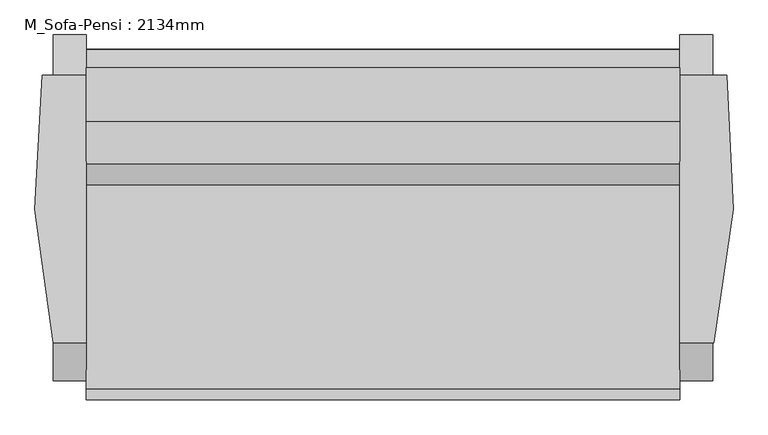
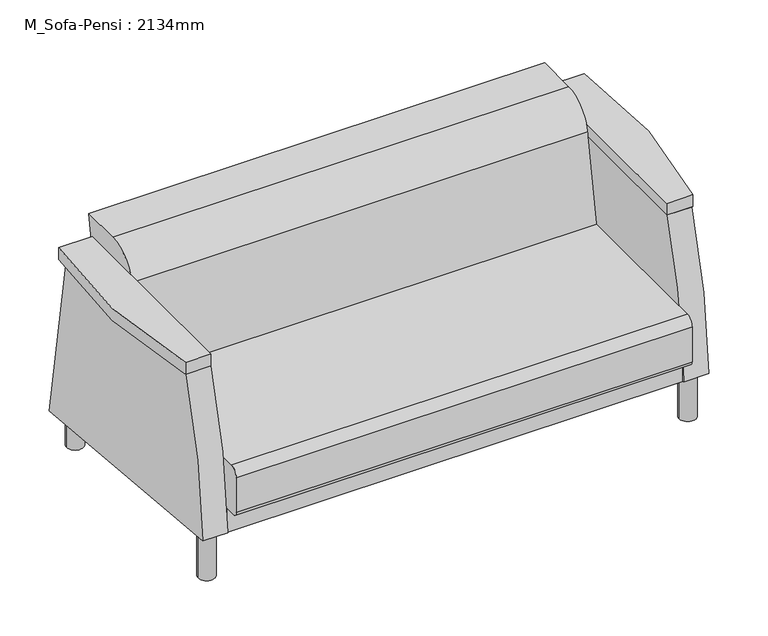
"""IFC4 building model written with IfcOpenShell, lengths in millimetres: furniture geometry, M_Sofa-Pensi : 2134mm."""

from ifc_helpers import new_model, si_unit, point, frame, frame_2d, origin, origin_with_axes, place, context, project, spatial, polyline, circle_curve, trimmed, segment, composite_curve, outline, extrude, source, transform, mapped, element, save
from ifc_brep_helpers import plane_surface, cylinder_surface, advanced_brep


def m_sofa_pensi_2134mm_8f487940(model_context):
    return source(origin(), model_context, "Body", "SolidModel", [
        advanced_brep(
        [(1040.60625, 701.7619204, 79.3588346), (1040.60625, 608.6917937, 626.0203985), (1040.60625, -9.3943348, 626.0203985), (1040.60625, -97.7900405, 149.3105671), (964.40625, -9.3943348, 626.0203985), (964.40625, 608.6917937, 626.0203985), (964.40625, 701.7619204, 79.3588346), (964.40625, -83.3930704, 148.0509954), (964.40625, 668.3047863, 148.0509954), (964.40625, 668.3047863, 224.2509954), (964.40625, -93.6952137, 224.2509954), (964.40625, -93.6952137, 148.9523161), (964.40625, -97.7900405, 149.3105671), (964.40625, -93.6952137, 148.0509954), (-407.19375, -83.3930704, 148.0509954), (-407.19375, -93.6952137, 148.0509954), (-407.19375, -93.6952137, 148.9523161), (-407.19375, 668.3047863, 224.2509954), (-407.19375, -93.6952137, 224.2509954), (-407.19375, 668.3047863, 148.0509954), (-407.19375, 701.7619204, 79.3588346), (-407.19375, 608.6917937, 626.0203985), (-407.19375, -9.3943348, 626.0203985), (-407.19375, -97.7900405, 149.3105671), (-483.39375, -9.3943348, 626.0203985), (-483.39375, 608.6917937, 626.0203985), (-483.39375, 701.7619204, 79.3588346), (-483.39375, -97.7900405, 149.3105671)],
        [
            (0, 1),
            (1, 2),
            (2, 3, circle_curve(frame((1040.60625, 1499.9783711, 99.5888442), z_axis=(1.0, 0.0, 0.0), x_axis=(0.0, 1.0, 0.0)), 1598.5418814)),
            (3, 0),
            (4, 5),
            (5, 6),
            (6, 7),
            (7, 8),
            (8, 9),
            (9, 10),
            (10, 4, circle_curve(frame((964.40625, 1499.9783711, 99.5888442), z_axis=(-1.0, 0.0, 0.0), x_axis=(0.0, 1.0, 0.0)), 1598.5418814)),
            (11, 12),
            (12, 10, circle_curve(frame((964.40625, 1499.9783711, 99.5888442), z_axis=(-1.0, 0.0, 0.0), x_axis=(0.0, 1.0, 0.0)), 1598.5418814)),
            (10, 11),
            (0, 6),
            (5, 1),
            (4, 2),
            (12, 3),
            (11, 7),
            (11, 13),
            (13, 7),
            (14, 15),
            (15, 16),
            (16, 14),
            (9, 17),
            (17, 18),
            (18, 10),
            (18, 16),
            (15, 13),
            (14, 19),
            (19, 8),
            (19, 17),
            (20, 21),
            (21, 22),
            (22, 18, circle_curve(frame((-407.19375, 1499.9783711, 99.5888442), z_axis=(1.0, 0.0, 0.0), x_axis=(0.0, 1.0, 0.0)), 1598.5418814)),
            (14, 20),
            (18, 23, circle_curve(frame((-407.19375, 1499.9783711, 99.5888442), z_axis=(1.0, 0.0, 0.0), x_axis=(0.0, 1.0, 0.0)), 1598.5418814)),
            (23, 16),
            (24, 25),
            (25, 26),
            (26, 27),
            (27, 24, circle_curve(frame((-483.39375, 1499.9783711, 99.5888442), z_axis=(-1.0, 0.0, 0.0), x_axis=(0.0, 1.0, 0.0)), 1598.5418814)),
            (27, 23),
            (22, 24),
            (26, 20),
            (25, 21),
        ],
        [
            plane_surface(frame((1040.60625, 608.6917937, 626.0203985), z_axis=(1.0000000000000002, 0.0, 0.0), x_axis=(0.0, -0.16783676484789783, 0.985814800236531))),
            plane_surface(frame((964.40625, 608.6917937, 626.0203985), z_axis=(-1.0000000000000002, 0.0, 0.0), x_axis=(0.0, 0.16783676484789783, -0.985814800236531))),
            plane_surface(frame((1040.60625, 701.7619204, 79.3588346), z_axis=(0.0, 0.985814800236531, 0.16783676484789783), x_axis=(-1.0, 0.0, 0.0))),
            plane_surface(frame((1040.60625, 608.6917937, 626.0203985), z_axis=(0.0, 0.0, 1.0), x_axis=(-1.0, 0.0, 0.0))),
            cylinder_surface(frame((964.40625, 1499.9783711, 99.5888442), z_axis=(1.0, 0.0, 0.0), x_axis=(0.0, 1.0, 0.0)), 1598.5418814),
            plane_surface(frame((1040.60625, -97.7900405, 149.3105671), z_axis=(0.0, -0.08715574274767213, -0.9961946980917444), x_axis=(-1.0, 0.0, 0.0))),
            plane_surface(frame((964.40625, -93.6952137, 224.2509954), z_axis=(1.0, 0.0, 0.0), x_axis=(0.0, -1.0, 0.0))),
            plane_surface(frame((-407.19375, -93.6952137, 224.2509954), z_axis=(-1.0, 0.0, 0.0), x_axis=(0.0, 1.0, 0.0))),
            plane_surface(frame((964.40625, 668.3047863, 224.2509954), z_axis=(0.0, 0.0, 1.0), x_axis=(-1.0, 0.0, 0.0))),
            plane_surface(frame((964.40625, -93.6952137, 224.2509954), z_axis=(0.0, -1.0, 0.0), x_axis=(-1.0, 0.0, 0.0))),
            plane_surface(frame((964.40625, -93.6952137, 148.0509954), z_axis=(0.0, 0.0, -1.0), x_axis=(-1.0, 0.0, 0.0))),
            plane_surface(frame((964.40625, 668.3047863, 148.0509954), z_axis=(0.0, 1.0, 0.0), x_axis=(-1.0, 0.0, 0.0))),
            plane_surface(frame((-407.19375, 3098.5202525, 99.5888442), z_axis=(1.0, 0.0, 0.0), x_axis=(0.0, 0.0, 1.0))),
            plane_surface(frame((-483.39375, 3098.5202525, 99.5888442), z_axis=(-1.0, 0.0, 0.0), x_axis=(0.0, 0.0, -1.0))),
            cylinder_surface(frame((-483.39375, 1499.9783711, 99.5888442), z_axis=(1.0, 0.0, 0.0), x_axis=(0.0, 1.0, 0.0)), 1598.5418814),
            plane_surface(frame((-407.19375, -97.7900405, 149.3105671), z_axis=(0.0, -0.08715574274766119, -0.9961946980917453), x_axis=(-1.0, 0.0, 0.0))),
            plane_surface(frame((-407.19375, 701.7619204, 79.3588346), z_axis=(0.0, 0.9858148002365317, 0.16783676484789398), x_axis=(-1.0, 0.0, 0.0))),
            plane_surface(frame((-407.19375, 608.6917937, 626.0203985), z_axis=(0.0, 0.0, 1.0), x_axis=(-1.0, 0.0, 0.0))),
        ],
        [
            (0, [[1, 2, 3, 4]]),
            (1, [[5, 6, 7, 8, 9, 10, 11]]),
            (1, [[12, 13, 14]]),
            (2, [[-1, 15, -6, 16]]),
            (3, [[-2, -16, -5, 17]]),
            (4, [[-3, -17, -11, -13, 18]]),
            (5, [[-4, -18, -12, 19, -7, -15]]),
            (6, [[20, 21, -19]]),
            (7, [[22, 23, 24]]),
            (8, [[25, 26, 27, -10]]),
            (9, [[-27, 28, -23, 29, -20, -14]]),
            (10, [[-29, -22, 30, 31, -8, -21]]),
            (11, [[-25, -9, -31, 32]]),
            (12, [[33, 34, 35, -26, -32, -30, 36]]),
            (12, [[37, 38, -28]]),
            (13, [[39, 40, 41, 42]]),
            (14, [[-42, 43, -37, -35, 44]]),
            (15, [[-41, 45, -36, -24, -38, -43]]),
            (16, [[-33, -45, -40, 46]]),
            (17, [[-34, -46, -39, -44]]),
        ],
    ),
        extrude(outline(composite_curve([segment(trimmed(circle_curve(frame_2d((-445.29375, -53.0901639)), 25.4), [point((-470.69375, -53.0901639))], [point((-419.89375, -53.0901639))], False, "CARTESIAN"), True, "CONTINUOUS"), segment(trimmed(circle_curve(frame_2d((-445.29375, -53.0901639)), 25.4), [point((-419.89375, -53.0901639))], [point((-470.69375, -53.0901639))], False, "CARTESIAN"), True, "CONTINUOUS")], self_intersect=False)), origin_with_axes(), (0.0, 0.0, 1.0), 148.43125),
        extrude(outline(composite_curve([segment(trimmed(circle_curve(frame_2d((-445.29375, 632.7098361)), 25.4), [point((-470.69375, 632.7098361))], [point((-419.89375, 632.7098361))], False, "CARTESIAN"), True, "CONTINUOUS"), segment(trimmed(circle_curve(frame_2d((-445.29375, 632.7098361)), 25.4), [point((-419.89375, 632.7098361))], [point((-470.69375, 632.7098361))], False, "CARTESIAN"), True, "CONTINUOUS")], self_intersect=False)), origin_with_axes(), (0.0, 0.0, 1.0), 148.43125),
        extrude(outline(composite_curve([segment(trimmed(circle_curve(frame_2d((1002.50625, 632.7098361)), 25.4), [point((977.10625, 632.7098361))], [point((1027.90625, 632.7098361))], False, "CARTESIAN"), True, "CONTINUOUS"), segment(trimmed(circle_curve(frame_2d((1002.50625, 632.7098361)), 25.4), [point((1027.90625, 632.7098361))], [point((977.10625, 632.7098361))], False, "CARTESIAN"), True, "CONTINUOUS")], self_intersect=False)), origin_with_axes(), (0.0, 0.0, 1.0), 148.43125),
        extrude(outline(composite_curve([segment(trimmed(circle_curve(frame_2d((1002.50625, -53.0901639)), 25.4), [point((977.10625, -53.0901639))], [point((1027.90625, -53.0901639))], False, "CARTESIAN"), True, "CONTINUOUS"), segment(trimmed(circle_curve(frame_2d((1002.50625, -53.0901639)), 25.4), [point((1027.90625, -53.0901639))], [point((977.10625, -53.0901639))], False, "CARTESIAN"), True, "CONTINUOUS")], self_intersect=False)), origin_with_axes(), (0.0, 0.0, 1.0), 148.43125),
        extrude(outline(composite_curve([segment(trimmed(circle_curve(frame_2d((-116.5901639, 351.2509954)), 25.4), [point((-141.9901639, 351.2509954))], [point((-116.5901639, 376.6509954))], False, "CARTESIAN"), True, "CONTINUOUS"), segment(polyline([(-116.5901639, 376.6509954), (355.3895541, 376.6509954), (402.1988177, 642.1195211)]), True, "CONTINUOUS"), segment(trimmed(circle_curve(frame_2d((502.2552854, 624.4768662)), 101.6), [point((402.1988177, 642.1195211))], [point((502.2552854, 726.0768662))], False, "CARTESIAN"), True, "CONTINUOUS"), segment(polyline([(502.2552854, 726.0768662), (626.3344485, 726.0768662), (609.5377828, 620.1719187), (667.6541767, 224.2509954), (-126.1151639, 224.2509954)]), True, "CONTINUOUS"), segment(trimmed(circle_curve(frame_2d((-126.1151639, 240.1259954)), 15.875), [point((-126.1151639, 224.2509954))], [point((-141.9901639, 240.1259954))], False, "CARTESIAN"), True, "CONTINUOUS"), segment(polyline([(-141.9901639, 240.1259954), (-141.9901639, 351.2509954)]), True, "CONTINUOUS")], self_intersect=False)), frame((-407.19375, 0.0, 0.0), z_axis=(1.0, 0.0, 0.0), x_axis=(0.0, 1.0, 0.0)), (0.0, 0.0, 1.0), 1371.6),
        extrude(outline(composite_curve([segment(polyline([(-407.19375, -9.3943348), (-483.39375, -9.3943348)]), True, "CONTINUOUS"), segment(trimmed(circle_curve(frame_2d((1074.7527561, 364.2020325)), 1602.3092024), [point((-483.39375, -9.3943348))], [point((-508.79375, 608.6917935))], False, "CARTESIAN"), True, "CONTINUOUS"), segment(polyline([(-508.79375, 608.6917935), (-407.19375, 608.6917935), (-407.19375, -9.3943348)]), True, "CONTINUOUS")], self_intersect=False)), frame((0.0, 0.0, 626.0203985), z_axis=(0.0, 0.0, 1.0), x_axis=(1.0, 0.0, 0.0)), (0.0, 0.0, 1.0), 38.1),
        extrude(outline(composite_curve([segment(polyline([(964.40625, -9.3943348), (964.40625, 608.9395268), (1073.0864453, 608.9395268)]), True, "CONTINUOUS"), segment(trimmed(circle_curve(frame_2d((-516.5771494, 377.0770652)), 1606.4839076), [point((1073.0864453, 608.9395268))], [point((1042.7273117, -9.3943348))], False, "CARTESIAN"), True, "CONTINUOUS"), segment(polyline([(1042.7273117, -9.3943348), (964.40625, -9.3943348)]), True, "CONTINUOUS")], self_intersect=False)), frame((0.0, 0.0, 626.0203985), z_axis=(0.0, 0.0, 1.0), x_axis=(1.0, 0.0, 0.0)), (0.0, 0.0, 1.0), 38.1),
    ])


if __name__ == "__main__":
    model = new_model("IFC4")
    model_context = context("Model", 3, world=origin())
    ifc_project = project(units=[si_unit("LENGTHUNIT", "METRE", prefix="MILLI")], contexts=[model_context])
    site = spatial("IfcSite", under=ifc_project)
    building = spatial("IfcBuilding", under=site)
    placement = place(None, origin())
    m_sofa_pensi_2134mm_shape = m_sofa_pensi_2134mm_8f487940(model_context)
    element("IfcFurniture", 1, ObjectType="M_Sofa-Pensi : 2134mm", at=placement, inside=building, context=model_context, shape_type="MappedRepresentation", body=[
        mapped(m_sofa_pensi_2134mm_shape, transform((0.0, 0.0, 0.0), x_axis=(1.0, 0.0, 0.0), y_axis=(0.0, 1.0, 0.0), z_axis=(0.0, 0.0, 1.0))),
    ])
    save(model, "model.ifc")

# Revit data of these elements
# Type "M_Sofa-Pensi : 2134mm"
#   Length = 5' - 0"
#   Sofa Material = Linen, Beige
#   Frame Material = Steel, Chrome Plated
#   Default Elevation = 0
# Element 1 (IfcFurniture, "M_Sofa-Pensi : 2134mm")
#   Materials on its faces: "Linen, Beige", "Steel, Chrome Plated"
# Materials
#   "Linen, Beige": class "Textile", colour RGB 249 239 230, transparency 0, Description = "Linen, beige", Cost = 0
#   "Steel, Chrome Plated": class "Metal", colour RGB 17 17 17, transparency 0, Description = "Chromiuim plated steel", Cost = 0
